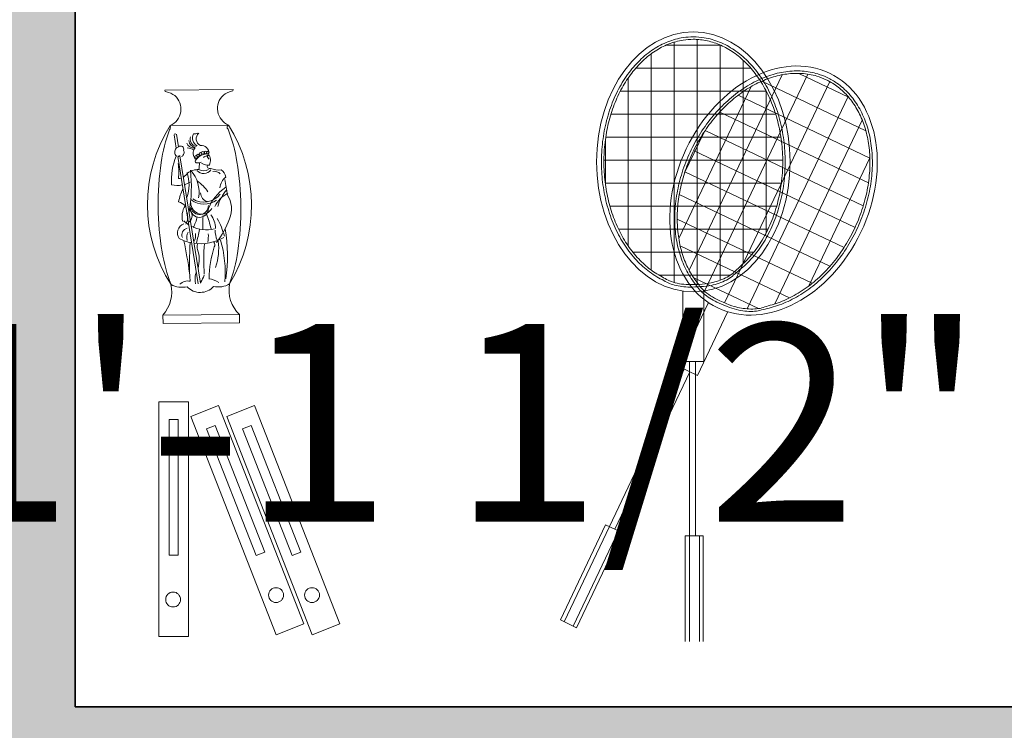
# Model space of a CAD drawing. Units: inches. Extents: x 638 to 1303, y 1 to 699.
# Tile 14 of 21: x 924 to 964, y 548 to 577. Entities that reach past the tile are written whole.
import ezdxf

# ---------------------------------------------------------------- set-up
doc = ezdxf.new("R2010")
doc.units = ezdxf.units.IN
doc.header["$MEASUREMENT"] = 0
for name, color, linetype, lineweight in [('A-ANNO-DIMS', 2, 'Continuous', 18), ('A-FURN-ACCS', 8, 'Continuous', 13), ('A-WALL', 7, 'Continuous', 35)]:
    doc.layers.add(name, color=color, linetype=linetype, lineweight=lineweight)
doc.layers.add('A-WALL-PATT', color=143, linetype='Continuous', lineweight=13, true_color=0x7aafdf)
doc.styles.get("Standard").update_dxf_attribs({"font": 'arial.ttf'})
doc.dimstyles.get("Standard").update_dxf_attribs({"dimtxt": 8, "dimasz": 0.18, "dimexe": 0.18, "dimexo": 0.0625, "dimgap": 0.09, "dimtad": 0, "dimtih": 1, "dimtoh": 1, "dimdec": 4, "dimzin": 0, "dimdsep": 46, "dimlunit": 3, "dimtxsty": 'Standard', "dimcen": 0.09, "dimadec": 0, "dimazin": 0, "dimtfac": 1, "dimtdec": 4, "dimtofl": 0, "dimtmove": 0, "dimatfit": 3, "dimfxl": 1, "dimtolj": 1, "dimtzin": 0, "dimarcsym": 0})

# ---------------------------------------------------------------- blocks, each defined once
blk = doc.blocks.new('*D68')
at = {"layer": 'A-ANNO-DIMS', "color": 0, "lineweight": -2, "transparency": 16777216}
for p, q in [((908.943, 524.881), (908.943, 560.499)), ((909.123, 560.319), (922.058, 560.319)), ((922.238, 524.881), (922.238, 560.499)), ((922.238, 560.319), (922.418, 560.319))]:
    blk.add_line(p, q, dxfattribs=at)
at = {"layer": 'A-ANNO-DIMS', "color": 0, "transparency": 16777216}
for points in [[(909.123, 560.349), (909.123, 560.289), (908.943, 560.319)], [(922.058, 560.349), (922.058, 560.289), (922.238, 560.319)]]:
    blk.add_solid(points, dxfattribs=at)
at = {"layer": 'Defpoints', "color": 0, "transparency": 16777216}
for p in [(922.238, 560.319), (908.943, 524.819), (922.238, 524.819)]:
    blk.add_point(p, dxfattribs=at)
at = {"layer": 'A-ANNO-DIMS', "color": 0, "transparency": 16777216, "insert": (942.085, 560.319), "char_height": 8, "attachment_point": 5}
blk.add_mtext('\\A1;1\'-1 1/2"', dxfattribs=at)

msp = doc.modelspace()

# ---------------------------------------------------------------- hatches: boundary and pattern name
at = {"layer": 'A-WALL-PATT'}
h = msp.add_hatch(color=256, dxfattribs=at)
h.dxf.hatch_style = 1
h.paths.add_polyline_path([(973.34524, 629.81895), (793.35541, 629.81895), (793.35541, 620.81895), (850.23798, 620.81895), (922.23798, 620.81895), (922.23798, 524.81895), (908.94335, 524.81895), (908.94335, 520.31895), (926.73798, 520.31895), (926.73798, 544.31895), (979.3571, 544.31895), (979.3571, 548.81895), (926.73798, 548.81895), (926.73798, 620.81895), (973.34524, 620.81895)])
h.paths.add_polyline_path([(758.35541, 629.81895), (697.23798, 629.81895), (697.23798, 586.77451), (706.23798, 586.77451), (706.23798, 620.81895), (758.35541, 620.81895)])
h.paths.add_polyline_path([(1075.85281, 629.81895), (1003.34524, 629.81895), (1003.34524, 620.81895), (1046.73798, 620.81895), (1046.73798, 560.81895), (1046.73798, 548.81895), (1026.3571, 548.81895), (1026.3571, 544.31895), (1046.73798, 544.31895), (1046.73798, 486.87457), (1051.23798, 486.87457), (1051.23798, 556.31895), (1162.89753, 556.31895), (1162.89753, 560.81895), (1051.23798, 560.81895), (1051.23798, 620.81895), (1075.85281, 620.81895)])
h.paths.add_polyline_path([(1228.23798, 629.81895), (1105.85281, 629.81895), (1105.85281, 620.81895), (1219.23798, 620.81895), (1219.23798, 560.81895), (1197.89753, 560.81895), (1197.89753, 556.31895), (1219.23798, 556.31895), (1219.23798, 498.80084), (1228.23798, 498.80084)])
h.paths.add_polyline_path([(1051.23798, 439.87457), (1046.73798, 439.87457), (1046.73798, 407.81895), (1219.23798, 407.81895), (1219.23798, 381.66175), (1228.23798, 381.66175), (1228.23798, 451.80084), (1219.23798, 451.80084), (1219.23798, 412.31895), (1051.23798, 412.31895)])
h.paths.add_polyline_path([(1228.23798, 346.66175), (1219.23798, 346.66175), (1219.23798, 335.81895), (1046.73798, 335.81895), (1046.73798, 273.56895), (1051.23798, 273.56895), (1051.23798, 331.31895), (1219.23798, 331.31895), (1219.23798, 308.99654), (1228.23798, 308.99654)])
h.paths.add_polyline_path([(1228.23798, 261.99654), (1219.23798, 261.99654), (1219.23798, 211.31895), (1051.23798, 211.31895), (1051.23798, 226.56895), (1046.73798, 226.56895), (1046.73798, 211.31895), (983.84714, 211.31895), (983.84714, 206.81895), (1219.23798, 206.81895), (1219.23798, 166.83987), (1228.23798, 166.83987)])
h.paths.add_polyline_path([(1228.23798, 119.83987), (1219.23798, 119.83987), (1219.23798, 50.81895), (1197.89277, 50.81895), (1197.89277, 41.81895), (1228.23798, 41.81895)])
h.paths.add_polyline_path([(1162.89277, 50.81895), (1069.02949, 50.81895), (1069.02949, 41.81895), (1162.89277, 41.81895)])
h.paths.add_polyline_path([(1010.02949, 50.81895), (941.89631, 50.81895), (917.77455, 50.81895), (917.77455, 41.81895), (941.89631, 41.81895), (1010.02949, 41.81895)])
h.paths.add_polyline_path([(882.77455, 50.81895), (854.73798, 50.81895), (854.73798, 145.50379), (850.23798, 145.50379), (850.23798, 50.81895), (793.49755, 50.81895), (793.49755, 41.81895), (882.77455, 41.81895)])
h.paths.add_polyline_path([(746.49755, 50.81895), (706.23798, 50.81895), (706.23798, 96.57416), (697.23798, 96.57416), (697.23798, 41.81895), (746.49755, 41.81895)])
h.paths.add_polyline_path([(706.23798, 206.81895), (714.01165, 206.81895), (714.01165, 211.31895), (706.23798, 211.31895), (706.23798, 251.21966), (697.23798, 251.21966), (697.23798, 143.57416), (706.23798, 143.57416)])
h.paths.add_polyline_path([(923.84714, 211.31895), (854.73798, 211.31895), (854.73798, 397.8313), (850.23798, 397.8313), (850.23798, 388.31895), (747.9539, 388.31895), (747.9539, 383.81895), (850.23798, 383.81895), (850.23798, 311.81895), (706.23798, 311.81895), (706.23798, 342.78787), (697.23798, 342.78787), (697.23798, 281.21966), (706.23798, 281.21966), (706.23798, 307.31895), (850.23798, 307.31895), (850.23798, 211.31895), (749.01165, 211.31895), (749.01165, 206.81895), (850.23798, 206.81895), (850.23798, 192.50379), (854.73798, 192.50379), (854.73798, 206.81895), (923.84714, 206.81895)])
h.paths.add_polyline_path([(706.23798, 434.70471), (697.23798, 434.70471), (697.23798, 372.78787), (706.23798, 372.78787), (706.23798, 383.81895), (712.9539, 383.81895), (712.9539, 388.31895), (706.23798, 388.31895)])
h.paths.add_polyline_path([(706.23798, 520.31895), (850.23798, 520.31895), (850.23798, 444.8313), (854.73798, 444.8313), (854.73798, 520.31895), (861.94335, 520.31895), (861.94335, 524.81895), (706.23798, 524.81895), (706.23798, 551.77451), (697.23798, 551.77451), (697.23798, 481.70471), (706.23798, 481.70471)])

# ---------------------------------------------------------------- linework, layer by layer
at = {"layer": 'A-FURN-ACCS'}
for p, q in [((951.92482, 565.92116), (951.92482, 575.84384)), ((952.88104, 575.60577), (950.65092, 575.60577)), ((950.9947, 566.0011), (950.9947, 575.73391)), ((952.85493, 566.09836), (952.85493, 575.61728)), ((950.06458, 566.50307), (950.06458, 575.26317)), ((953.78505, 566.76477), (953.78505, 575.00102)), ((954.09923, 574.67566), (949.43274, 574.67566)), ((949.13447, 567.4772), (949.13447, 574.28904)), ((951.5981, 566.50206), (955.36223, 574.41221)), ((952.22228, 565.64913), (956.40438, 574.43761)), ((958.05264, 573.51137), (956.03889, 574.46963)), ((930.36629, 573.79273, 3.93985), (933.1319, 573.82098, 3.93985)), ((951.1768, 567.78134), (954.10378, 573.93226)), ((953.0278, 565.17728), (957.29149, 574.13722)), ((958.75298, 572.14805), (954.53924, 574.1532)), ((954.7224, 573.74554), (948.80958, 573.74554)), ((958.91602, 571.04041), (953.57688, 573.58109)), ((953.94381, 564.93762), (958.03401, 573.53297)), ((954.71517, 568.00675), (954.71517, 573.75949)), ((955.10079, 572.81542), (948.4312, 572.81542)), ((958.85803, 570.03795), (952.83555, 572.90381)), ((955.07004, 565.13971), (958.60908, 572.57684)), ((932.94155, 572.37729, 3.93985), (930.58608, 572.35324, 3.93985)), ((930.73828, 572.00632, 3.93985), (930.81707, 572.02686, 3.93985)), ((930.73848, 571.98658, 3.93985), (930.82557, 571.44523, 3.93985)), ((930.83702, 572.00733, 3.93985), (930.92035, 571.48941, 3.93985)), ((948.20435, 569.98468), (948.20435, 571.78156)), ((955.31279, 571.88531), (948.21919, 571.88531)), ((951.41437, 570.44519), (952.18647, 572.06773)), ((958.6498, 569.10698), (952.24445, 572.15503)), ((930.94371, 571.51169, 3.93985), (930.91472, 571.52437, 3.93985)), ((930.88613, 571.1049, 3.93985), (931.71527, 565.95114, 3.93985)), ((930.97802, 571.13095, 3.93985), (931.80716, 565.9772, 3.93985)), ((958.31746, 568.23507), (951.77746, 571.3472)), ((956.44358, 565.86153), (958.91548, 571.05612)), ((955.38734, 570.95519), (948.14463, 570.95519)), ((957.86867, 567.41857), (951.42692, 570.48395)), ((955.33294, 570.02507), (948.19903, 570.02507)), ((957.29791, 566.66012), (951.19835, 569.56266)), ((955.14346, 569.09496), (948.38851, 569.09496)), ((956.58277, 565.97037), (951.11417, 568.57266)), ((954.79409, 568.16484), (948.73789, 568.16484)), ((955.66331, 565.37785), (951.2343, 567.48544)), ((954.21843, 567.23473), (949.31353, 567.23473)), ((953.27128, 566.30461), (950.36758, 566.30461)), ((954.40839, 564.94496), (951.78642, 566.19265)), ((951.33596, 565.63601), (951.33596, 562.79817)), ((952.19601, 565.63601), (952.19601, 562.79817)), ((952.37355, 565.17282), (951.15416, 562.61032)), ((930.28799, 564.68019, 3.93985), (933.39058, 564.71188, 3.93985)), ((930.28799, 564.68019, 3.93985), (930.29148, 564.33761, 3.93985)), ((933.39058, 564.71188, 3.93985), (933.39408, 564.3693, 3.93985)), ((953.15016, 564.80327), (951.93076, 562.24076)), ((930.29148, 564.33761, 3.93985), (933.39408, 564.3693, 3.93985)), ((951.15416, 562.61032), (951.93076, 562.24076)), ((951.33596, 562.79817), (952.19601, 562.79817)), ((951.60659, 562.79817), (951.60659, 555.74243)), ((951.85462, 562.79817), (951.85462, 555.74243)), ((951.39853, 562.49403), (948.36675, 556.12287)), ((951.6225, 562.38745), (948.59071, 556.01629)), ((930.11865, 551.67657), (930.11865, 561.1656)), ((930.11865, 561.1656), (931.32767, 561.1656)), ((931.32767, 561.1656), (931.32767, 551.67657)), ((931.41319, 560.57978), (932.53902, 561.02049)), ((932.53902, 561.02049), (935.99798, 552.18435)), ((932.87056, 560.57978), (933.99639, 561.02049)), ((933.99639, 561.02049), (937.45534, 552.18435)), ((930.91023, 560.46272), (930.53474, 560.46272)), ((930.53474, 560.46272), (930.53474, 554.96154)), ((930.91023, 554.96154), (930.91023, 560.46272)), ((934.87215, 551.74364), (931.41319, 560.57978)), ((932.40652, 560.21381), (932.05687, 560.07693)), ((934.41182, 555.09114), (932.40652, 560.21381)), ((936.32951, 551.74364), (932.87056, 560.57978)), ((933.86389, 560.21381), (933.51424, 560.07693)), ((935.86919, 555.09114), (933.86389, 560.21381)), ((932.05687, 560.07693), (934.06217, 554.95426)), ((933.51424, 560.07693), (935.51953, 554.95426)), ((946.38188, 552.34124), (948.21563, 556.19478)), ((948.36675, 556.12287), (946.533, 552.26932)), ((948.74148, 555.94455), (946.90773, 552.09101)), ((948.87502, 555.881), (947.04127, 552.02746)), ((948.21563, 556.19478), (948.87502, 555.881)), ((951.43923, 555.74243), (952.16948, 555.74243)), ((951.43923, 551.47483), (951.43923, 555.74243)), ((951.60659, 555.74243), (951.60659, 551.47483)), ((952.02159, 555.74243), (952.02159, 551.47483)), ((952.16948, 555.74243), (952.16948, 551.47483)), ((934.06217, 554.95426), (934.41182, 555.09114)), ((935.51953, 554.95426), (935.86919, 555.09114)), ((930.53474, 554.96154), (930.91023, 554.96154)), ((947.04127, 552.02746), (946.38188, 552.34124)), ((935.99798, 552.18435), (934.87215, 551.74364)), ((937.45534, 552.18435), (936.32951, 551.74364)), ((931.32767, 551.67657), (930.11865, 551.67657))]:
    msp.add_line(p, q, dxfattribs=at)
for centre, radius in [((931.63494, 571.08741, 3.93985), 0.05363), ((931.70144, 571.13832, 3.93985), 0.05363), ((931.80966, 571.20641, 3.93985), 0.05363), ((931.90138, 571.24921, 3.93985), 0.05363), ((932.01849, 571.26715, 3.93985), 0.05363), ((932.10234, 571.25963, 3.93985), 0.05363), ((930.70162, 553.16949), 0.30075), ((934.87081, 553.34635), 0.30075), ((936.32817, 553.34635), 0.30075)]:
    msp.add_circle(centre, radius, dxfattribs=at)
for centre, radius, start, end in [((930.4364, 573.78534, 3.93985), 0.0705, 173.978672, 263.589878), ((933.06195, 573.81215, 3.93985), 0.0705, 277.580483, 7.191689), ((930.28491, 572.92087, 3.93985), 0.80729, 53.36252, 79.752247), ((930.28893, 573.01851, 3.93985), 0.72862, 294.068985, 49.030396), ((933.22506, 573.0485, 3.93985), 0.72862, 132.139965, 247.101376), ((933.23107, 572.95097, 3.93985), 0.80729, 101.418114, 127.807841), ((935.62317, 569.16134, 3.93985), 5.96326, 147.63841, 212.934069), ((936.80547, 569.89792, 3.93985), 6.65759, 159.879075, 171.686697), ((930.38882, 572.30571, 3.93985), 0.20291, 324.592438, 13.5447), ((932.97842, 572.28989, 3.93985), 0.09486, 112.872738, 234.825052), ((926.72059, 569.79492, 3.93985), 6.65759, 9.483664, 21.291286), ((927.75237, 569.1267, 3.93985), 6.12323, 328.676594, 32.063754), ((931.69522, 571.8088, 3.93985), 0.30225, 161.219878, 257.602502), ((931.87895, 571.86156, 3.93985), 0.38896, 155.032994, 237.440628), ((931.5612, 572.48064, 3.93985), 0.45624, 265.618389, 288.22447), ((931.92349, 571.82059, 3.93985), 0.28985, 128.416535, 246.44791), ((930.98098, 571.28762, 3.93985), 0.21579, 135.652185, 231.313321), ((930.95315, 571.29534, 3.93985), 0.19683, 97.608952, 133.084254), ((930.98098, 571.28762, 3.93985), 0.21579, 106.065257, 106.543427), ((931.00569, 571.40497, 3.93985), 0.12341, 338.05295, 133.167285), ((931.53171, 571.7458, 3.93985), 0.29475, 199.396632, 277.795371), ((931.12423, 570.46778, 3.93985), 0.99454, 65.731284, 81.253778), ((931.64392, 571.7836, 3.93985), 0.31433, 186.612201, 260.351866), ((931.82188, 571.23685, 3.93985), 0.31662, 136.70467, 233.998908), ((931.8405, 571.24917, 3.93985), 0.30747, 355.07693, 96.129443), ((933.14517, 570.15203, 3.93985), 2.51236, 157.363881, 184.555163), ((930.97993, 571.0325, 3.93985), 0.09847, 89.36162, 156.718708), ((930.95336, 571.26832, 3.93985), 0.18978, 298.454265, 28.490298), ((932.07819, 570.66237, 3.93985), 0.54504, 82.744379, 144.264353), ((932.06575, 570.9381, 3.93985), 0.1872, 91.201601, 137.200919), ((932.11675, 571.07969, 3.93985), 0.07704, 68.214429, 135.562268), ((934.51128, 572.6537, 3.93985), 2.88286, 211.821697, 215.192011), ((932.05964, 571.22938, 3.93985), 0.10415, 271.201601, 317.867143), ((931.73216, 570.94371, 3.93985), 0.47858, 337.12838, 33.987651), ((941.79914, 569.16824, 3.93985), 11.70429, 171.686697, 180.58518), ((928.6136, 570.49435, 3.93985), 2.31828, 353.001994, 8.168367), ((931.72075, 569.84872, 3.93985), 0.72718, 88.448153, 126.557118), ((931.6521, 570.90935, 3.93985), 0.06058, 93.166791, 258.408226), ((931.70503, 571.17964, 3.93985), 0.33601, 258.827884, 292.582513), ((929.04284, 571.05801, 3.93985), 2.74039, 349.861746, 355.669622), ((931.93491, 570.87411, 3.93985), 0.35624, 236.915164, 304.255197), ((932.09995, 571.15217, 3.93985), 0.4012, 232.608356, 280.506503), ((932.18004, 570.71116, 3.93985), 0.09734, 151.975277, 290.43311), ((932.53204, 571.39072, 3.93985), 0.8338, 247.578924, 278.070792), ((921.74286, 568.96339, 3.93985), 11.70429, 0.58518, 9.483664), ((930.88011, 570.6955, 3.93985), 0.48483, 274.080429, 286.872559), ((930.88011, 570.6955, 3.93985), 0.48483, 299.139964, 327.195908), ((929.80227, 569.96272, 3.93985), 1.54504, 340.445867, 18.476457), ((925.46117, 569.90469, 3.93985), 5.97893, 349.800704, 6.219849), ((930.4197, 569.65847, 3.93985), 1.3323, 350.156464, 41.022084), ((931.93771, 570.78096, 3.93985), 0.36935, 221.679853, 323.437905), ((932.36689, 570.15732, 3.93985), 0.34925, 45.606962, 98.715113), ((933.20294, 569.79199, 3.93985), 0.60711, 127.916667, 176.002542), ((932.3963, 570.20722, 3.93985), 0.43822, 8.360591, 54.769096), ((930.85946, 571.10517, 3.93985), 1.17323, 259.256302, 280.143751), ((932.96614, 568.90138, 3.93985), 2.07389, 154.648215, 169.915004), ((930.85946, 571.10517, 3.93985), 1.17323, 285.066545, 296.896447), ((932.96614, 568.90138, 3.93985), 2.07389, 148.73, 150.009002), ((930.9778, 568.99161, 3.93985), 1.31647, 31.087903, 57.454033), ((933.82022, 568.33727, 3.93985), 1.81119, 122.987839, 160.524595), ((925.12396, 568.56865, 3.93985), 7.83324, 7.132694, 11.809959), ((931.94586, 570.07943, 3.93985), 0.82432, 236.908555, 322.51085), ((932.19048, 569.64425, 3.93985), 0.38143, 182.310148, 254.645077), ((933.51177, 568.50799, 3.93985), 1.26216, 118.1905, 152.943875), ((934.24623, 568.57152, 3.93985), 1.81371, 139.135045, 163.609661), ((932.00236, 568.98323, 3.93985), 1.06448, 337.449397, 32.874556), ((941.79914, 569.16824, 3.93985), 11.70429, 180.58518, 189.483664), ((930.68518, 568.5214, 3.93985), 0.78066, 48.563779, 72.163918), ((931.89881, 568.68176, 3.93985), 0.83406, 149.165045, 194.233015), ((931.76637, 569.00441, 3.93985), 0.36546, 181.777586, 359.392726), ((931.87408, 569.22743, 3.93985), 0.45567, 179.662937, 330.34047), ((931.77093, 569.11359, 3.93985), 0.3597, 192.9887, 0.854117), ((931.95684, 570.04499, 3.93985), 0.86894, 233.251607, 305.716721), ((921.74286, 568.96339, 3.93985), 11.70429, 351.686697, 0.58518), ((930.71438, 568.65661, 3.93985), 0.5779, 329.05964, 17.851904), ((931.1593, 568.70439, 3.93985), 0.31379, 302.464066, 58.706295), ((929.79658, 569.15693, 3.93985), 1.94875, 331.409171, 345.237839), ((937.06034, 568.31067, 3.93985), 5.15937, 175.427248, 181.790816), ((927.14768, 566.96975, 3.93985), 5.2315, 13.292723, 20.275302), ((931.38178, 568.15557, 3.93985), 1.0355, 2.135398, 34.693756), ((929.56809, 567.00685, 3.93985), 3.32443, 15.262978, 28.432739), ((931.27385, 568.00443, 3.93985), 0.40039, 110.925785, 213.353073), ((931.33295, 567.93208, 3.93985), 0.27715, 102.936106, 202.6875), ((932.05356, 569.49529, 3.93985), 1.36035, 227.22056, 237.889319), ((932.05356, 569.49529, 3.93985), 1.36035, 243.009854, 283.765708), ((929.0917, 570.0943, 3.93985), 4.17966, 323.739259, 338.684771), ((931.81216, 569.49248, 3.93985), 1.91823, 242.936433, 259.073084), ((931.59793, 567.8441, 3.93985), 0.34926, 144.945369, 202.796846), ((931.14157, 567.91686, 3.93985), 0.47275, 325.954787, 8.718551), ((931.81216, 569.49248, 3.93985), 1.91823, 262.062534, 299.478659), ((-1212959.28846, 247911.29423, 3.93985), 1238834.17867, 348.48301372545, 348.48303986891), ((930.94009, 567.86326, 3.93985), 1.18763, 349.081374, 5.351792), ((933.76784, 568.1981, 3.93985), 1.37275, 183.470149, 200.333874), ((926.50054, 567.09745, 3.93985), 6.40311, 351.45087, 9.71949), ((909.96653, 563.26358, 3.93985), 21.62867, 8.303796, 11.802898), ((941.70043, 566.81783, 3.93985), 10.33722, 175.488003, 184.249156), ((931.97939, 567.44949, 3.93985), 0.30591, 159.799983, 201.370377), ((940.3671, 566.90825, 3.93985), 8.42516, 175.44269, 183.907751), ((936.68024, 566.09932, 3.93985), 4.51979, 162.697804, 179.250289), ((932.23917, 567.52946, 3.93985), 0.15233, 325.674824, 46.923716), ((930.45468, 567.35144, 3.93985), 2.09214, 339.390871, 9.091232), ((928.17324, 566.40591, 3.93985), 4.6365, 355.309359, 16.496738), ((936.82141, 568.33671, 3.93985), 6.65759, 189.483664, 201.291286), ((930.47506, 566.93868, 3.93985), 1.28317, 344.089179, 18.132248), ((926.73654, 568.2337, 3.93985), 6.65759, 339.879075, 351.686697), ((932.34974, 566.13539, 3.93985), 0.76143, 162.04486, 193.669528), ((930.47506, 566.93868, 3.93985), 1.28317, 333.698527, 335.445092), ((83932.43772, -39905.60547, 3.93985), 92342.04718, 154.0056530881, 154.0058448081), ((929.20436, 565.6302, 3.93985), 1.4411, 318.759111, 12.038114), ((931.06593, 566.75648, 3.93985), 0.9494, 241.863974, 282.544569), ((931.28714, 565.64577, 3.93985), 0.41937, 75.573225, 137.468871), ((931.79904, 566.32053, 3.93985), 0.72006, 222.967172, 270.58518), ((931.79904, 566.32053, 3.93985), 0.72006, 270.58518, 318.203188), ((931.96493, 565.04008, 3.93985), 1.13197, 58.43802, 81.047436), ((932.52309, 566.77137, 3.93985), 0.9494, 258.625792, 299.306386), ((934.28094, 565.68472, 3.93985), 1.31878, 168.684615, 227.534507)]:
    msp.add_arc(centre, radius, start, end, dxfattribs=at)
for centre, major_axis in [((951.76598, 570.88312), (0, 5.26318)), ((955.01649, 569.72606), (2.26154, 4.75252))]:
    msp.add_ellipse(centre, major_axis=major_axis, ratio=0.74468092, dxfattribs=at)
for points, knots in [([(951.76598, 575.94787), (951.62974, 575.94787), (951.49349, 575.93763), (951.1486, 575.88559), (950.94092, 575.82962), (950.53439, 575.66984), (950.33554, 575.56603), (949.95255, 575.31279), (949.76842, 575.16336), (949.42077, 574.82271), (949.25727, 574.6315), (948.95634, 574.21275), (948.81892, 573.98521), (948.57479, 573.50061), (948.46809, 573.24356), (948.28899, 572.70779), (948.21659, 572.42908), (948.10851, 571.85858), (948.07283, 571.5668), (948.03938, 570.9792), (948.04161, 570.68338), (948.0839, 570.09684), (948.12397, 569.80614), (948.2406, 569.23881), (948.31717, 568.96221), (948.50424, 568.4316), (948.61475, 568.17762), (948.86599, 567.70001), (949.00672, 567.4764), (949.31367, 567.06622), (949.47989, 566.87965), (949.83228, 566.54882), (950.01844, 566.40456), (950.4048, 566.16201), (950.60498, 566.06372), (950.8895, 565.91514), (951.09784, 565.86485), (951.51726, 565.81308), (951.72835, 565.8116), (952.39612, 565.85745), (952.60478, 565.9048), (953.01428, 566.04756), (953.21512, 566.14299), (953.47914, 566.37997), (953.66633, 566.52152), (954.02111, 566.84722), (954.1887, 567.03136), (954.49872, 567.43705), (954.64114, 567.65859), (954.89602, 568.13249), (955.00848, 568.38484), (955.19965, 568.91268), (955.27835, 569.18815), (955.39939, 569.75374), (955.44172, 570.04384), (955.48859, 570.62973), (955.49313, 570.9255), (955.46427, 571.51356), (955.43087, 571.80584), (955.32724, 572.37788), (955.25701, 572.65764), (955.08206, 573.196), (954.97735, 573.4546), (954.73695, 573.94274), (954.60127, 574.17227), (954.30352, 574.59539), (954.14145, 574.78897), (953.79632, 575.13466), (953.61327, 575.28675), (953.23209, 575.5455), (953.03396, 575.65216), (952.62853, 575.81771), (952.42122, 575.87662), (952.064, 575.93562), (951.91499, 575.94787), (951.76598, 575.94787)], [0, 0, 0, 0, 0.11189338, 0.11189338, 0.2847196, 0.2847196, 0.45754582, 0.45754582, 0.63037204, 0.63037204, 0.80319826, 0.80319826, 0.97602448, 0.97602448, 1.1488507, 1.1488507, 1.32167692, 1.32167692, 1.49450315, 1.49450315, 1.66732937, 1.66732937, 1.84015559, 1.84015559, 2.01298181, 2.01298181, 2.18580803, 2.18580803, 2.35863425, 2.35863425, 2.53146047, 2.53146047, 2.70428669, 2.70428669, 2.87711291, 2.87711291, 3.04993914, 3.04993914, 3.22276536, 3.22276536, 3.39559158, 3.39559158, 3.5684178, 3.5684178, 3.74124402, 3.74124402, 3.91407024, 3.91407024, 4.08689646, 4.08689646, 4.25972268, 4.25972268, 4.4325489, 4.4325489, 4.60537513, 4.60537513, 4.77820135, 4.77820135, 4.95102757, 4.95102757, 5.12385379, 5.12385379, 5.29668001, 5.29668001, 5.46950623, 5.46950623, 5.64233245, 5.64233245, 5.81515867, 5.81515867, 5.98798489, 5.98798489, 6.16081112, 6.16081112, 6.28318531, 6.28318531, 6.28318531, 6.28318531]), ([(951.76598, 575.84866), (951.63014, 575.84866), (951.49428, 575.8381), (951.15487, 575.78508), (950.95211, 575.72907), (950.57178, 575.57625), (950.39349, 575.48331), (950.04801, 575.25882), (949.88081, 575.12714), (949.56253, 574.82786), (949.41145, 574.66018), (949.12993, 574.29282), (948.99952, 574.09308), (948.76333, 573.66667), (948.6576, 573.43996), (948.47399, 572.96557), (948.39616, 572.71789), (948.27076, 572.20818), (948.22321, 571.94619), (948.15981, 571.41491), (948.14398, 571.14568), (948.14452, 570.60723), (948.16087, 570.33805), (948.22532, 569.80702), (948.27337, 569.5452), (948.39978, 569.03597), (948.47808, 568.78858), (948.66261, 568.31489), (948.76878, 568.08857), (949.00578, 567.66306), (949.13658, 567.4638), (949.41877, 567.0975), (949.57017, 566.93039), (949.88724, 566.6339), (950.05278, 566.50408), (950.40991, 566.27253), (950.60254, 566.17427), (950.9059, 566.01083), (951.1421, 565.95457), (951.617, 565.90691), (952.1038, 565.91547), (952.53766, 565.99058), (952.73343, 566.04727), (953.11719, 566.20525), (953.30515, 566.30649), (953.54391, 566.55192), (953.7187, 566.69604), (954.04949, 567.02396), (954.20549, 567.20769), (954.49341, 567.60989), (954.62534, 567.82831), (954.86058, 568.2936), (954.96392, 568.54043), (955.13843, 569.05519), (955.20965, 569.3231), (955.3175, 569.87195), (955.35418, 570.15289), (955.39171, 570.71927), (955.39261, 571.00475), (955.35858, 571.57156), (955.32368, 571.85293), (955.2208, 572.3947), (955.15388, 572.65552), (954.98989, 573.15701), (954.89291, 573.39781), (954.67348, 573.85024), (954.55138, 574.06228), (954.28751, 574.45158), (954.14618, 574.62945), (953.84613, 574.95173), (953.6874, 575.09607), (953.35702, 575.34827), (953.1854, 575.45606), (952.83368, 575.63339), (952.65363, 575.70288), (952.28907, 575.80283), (952.1046, 575.8333), (951.86846, 575.84716), (951.81722, 575.84866), (951.76598, 575.84866)], [0, 0, 0, 0, 0.11579064, 0.11579064, 0.29073032, 0.29073032, 0.4507067, 0.4507067, 0.61090847, 0.61090847, 0.77111024, 0.77111024, 0.93131201, 0.93131201, 1.09151378, 1.09151378, 1.25171555, 1.25171555, 1.41191732, 1.41191732, 1.57211909, 1.57211909, 1.73232086, 1.73232086, 1.89252263, 1.89252263, 2.0527244, 2.0527244, 2.21292617, 2.21292617, 2.37312794, 2.37312794, 2.53332971, 2.53332971, 2.69180105, 2.69180105, 2.86418207, 2.86418207, 3.06698542, 3.06698542, 3.26978878, 3.26978878, 3.43901445, 3.43901445, 3.60824012, 3.60824012, 3.77746579, 3.77746579, 3.94669146, 3.94669146, 4.11591713, 4.11591713, 4.2851428, 4.2851428, 4.45436847, 4.45436847, 4.62359414, 4.62359414, 4.79281981, 4.79281981, 4.96204548, 4.96204548, 5.12614683, 5.12614683, 5.28969056, 5.28969056, 5.45084761, 5.45084761, 5.60858038, 5.60858038, 5.76631316, 5.76631316, 5.92404593, 5.92404593, 6.08177871, 6.08177871, 6.23951149, 6.23951149, 6.28318531, 6.28318531, 6.28318531, 6.28318531]), ([(957.19277, 574.29941), (957.06974, 574.35795), (956.94231, 574.40725), (956.60852, 574.50845), (956.39694, 574.54715), (955.9612, 574.57756), (955.73704, 574.56926), (955.28239, 574.50516), (955.05191, 574.44934), (954.59162, 574.29113), (954.36182, 574.18873), (953.91016, 573.93991), (953.6883, 573.7935), (953.25963, 573.46081), (953.05283, 573.27455), (952.66089, 572.86772), (952.47575, 572.64716), (952.13302, 572.17846), (951.97543, 571.93032), (951.69274, 571.4141), (951.56764, 571.14603), (951.3538, 570.59823), (951.26507, 570.31851), (951.12661, 569.75611), (951.07689, 569.47344), (951.01782, 568.91394), (951.00847, 568.63711), (951.03011, 568.09789), (951.06111, 567.8355), (951.16202, 567.33322), (951.23194, 567.09333), (951.40799, 566.64318), (951.5141, 566.43293), (951.75876, 566.0479), (951.89728, 565.87312), (952.09035, 565.61671), (952.25687, 565.48177), (952.61335, 565.25481), (952.80332, 565.16277), (953.426, 564.91724), (953.63476, 564.87033), (954.06588, 564.82328), (954.28823, 564.82315), (954.62847, 564.92369), (954.85832, 564.97108), (955.31863, 565.11273), (955.54908, 565.20699), (956.00334, 565.4401), (956.22713, 565.57895), (956.66092, 565.89736), (956.8709, 566.0769), (957.27032, 566.47138), (957.45976, 566.68631), (957.81209, 567.14501), (957.97496, 567.38878), (958.26903, 567.89768), (958.40022, 568.1628), (958.62684, 568.70621), (958.72227, 568.98448), (958.8745, 569.54555), (958.93129, 569.82834), (959.00465, 570.38964), (959.02121, 570.66815), (959.01389, 571.21222), (958.99001, 571.47778), (958.90295, 571.98779), (958.83979, 572.23223), (958.67668, 572.69267), (958.57675, 572.90866), (958.34373, 573.3061), (958.21065, 573.48754), (957.91569, 573.81125), (957.75382, 573.95352), (957.45661, 574.16029), (957.32732, 574.23538), (957.19277, 574.29941)], [0, 0, 0, 0, 0.11189338, 0.11189338, 0.2847196, 0.2847196, 0.45754582, 0.45754582, 0.63037204, 0.63037204, 0.80319826, 0.80319826, 0.97602448, 0.97602448, 1.1488507, 1.1488507, 1.32167692, 1.32167692, 1.49450315, 1.49450315, 1.66732937, 1.66732937, 1.84015559, 1.84015559, 2.01298181, 2.01298181, 2.18580803, 2.18580803, 2.35863425, 2.35863425, 2.53146047, 2.53146047, 2.70428669, 2.70428669, 2.87711291, 2.87711291, 3.04993914, 3.04993914, 3.22276536, 3.22276536, 3.39559158, 3.39559158, 3.5684178, 3.5684178, 3.74124402, 3.74124402, 3.91407024, 3.91407024, 4.08689646, 4.08689646, 4.25972268, 4.25972268, 4.4325489, 4.4325489, 4.60537513, 4.60537513, 4.77820135, 4.77820135, 4.95102757, 4.95102757, 5.12385379, 5.12385379, 5.29668001, 5.29668001, 5.46950623, 5.46950623, 5.64233245, 5.64233245, 5.81515867, 5.81515867, 5.98798489, 5.98798489, 6.16081112, 6.16081112, 6.28318531, 6.28318531, 6.28318531, 6.28318531]), ([(957.15014, 574.20982), (957.02747, 574.26819), (956.90025, 574.31703), (956.571, 574.415), (956.36385, 574.45155), (955.95475, 574.47698), (955.75382, 574.46967), (955.3454, 574.4154), (955.13784, 574.36835), (954.72184, 574.23487), (954.51337, 574.14837), (954.10131, 573.93763), (953.89773, 573.8133), (953.50123, 573.52975), (953.30834, 573.37047), (952.9387, 573.021), (952.76201, 572.83079), (952.42975, 572.42443), (952.27424, 572.20828), (951.98871, 571.75579), (951.85873, 571.51948), (951.62784, 571.03305), (951.52695, 570.78296), (951.35696, 570.27576), (951.28785, 570.01869), (951.18319, 569.50456), (951.14759, 569.24752), (951.11068, 568.7405), (951.1093, 568.49052), (951.14046, 568.00445), (951.17295, 567.76833), (951.27036, 567.31631), (951.33527, 567.10036), (951.49418, 566.69639), (951.58788, 566.50804), (951.81086, 566.1455), (951.94258, 565.97399), (952.14628, 565.69607), (952.33538, 565.54377), (952.74372, 565.29668), (953.18697, 565.09523), (953.61101, 564.97663), (953.81215, 564.9437), (954.22656, 564.92145), (954.43978, 564.93211), (954.76084, 565.05113), (954.98059, 565.10616), (955.42019, 565.26013), (955.64001, 565.35899), (956.07281, 565.59846), (956.2858, 565.73899), (956.69814, 566.05806), (956.89752, 566.23653), (957.27628, 566.62637), (957.45571, 566.83768), (957.78893, 567.28694), (957.94276, 567.52486), (958.22003, 568.02017), (958.34351, 568.27755), (958.55633, 568.80399), (958.64572, 569.07306), (958.78561, 569.60647), (958.83726, 569.87074), (958.90467, 570.39405), (958.92057, 570.65315), (958.91683, 571.15598), (958.89769, 571.39991), (958.8267, 571.86481), (958.77551, 572.08616), (958.64306, 572.5061), (958.56174, 572.70463), (958.37179, 573.07433), (958.26314, 573.2454), (958.02174, 573.55665), (957.88902, 573.69677), (957.60278, 573.94368), (957.4493, 574.05045), (957.24203, 574.16443), (957.1964, 574.1878), (957.15014, 574.20982)], [0, 0, 0, 0, 0.11579064, 0.11579064, 0.29073032, 0.29073032, 0.4507067, 0.4507067, 0.61090847, 0.61090847, 0.77111024, 0.77111024, 0.93131201, 0.93131201, 1.09151378, 1.09151378, 1.25171555, 1.25171555, 1.41191732, 1.41191732, 1.57211909, 1.57211909, 1.73232086, 1.73232086, 1.89252263, 1.89252263, 2.0527244, 2.0527244, 2.21292617, 2.21292617, 2.37312794, 2.37312794, 2.53332971, 2.53332971, 2.69180105, 2.69180105, 2.86418207, 2.86418207, 3.06698542, 3.06698542, 3.26978878, 3.26978878, 3.43901445, 3.43901445, 3.60824012, 3.60824012, 3.77746579, 3.77746579, 3.94669146, 3.94669146, 4.11591713, 4.11591713, 4.2851428, 4.2851428, 4.45436847, 4.45436847, 4.62359414, 4.62359414, 4.79281981, 4.79281981, 4.96204548, 4.96204548, 5.12614683, 5.12614683, 5.28969056, 5.28969056, 5.45084761, 5.45084761, 5.60858038, 5.60858038, 5.76631316, 5.76631316, 5.92404593, 5.92404593, 6.08177871, 6.08177871, 6.23951149, 6.23951149, 6.28318531, 6.28318531, 6.28318531, 6.28318531])]:
    msp.add_open_spline(points, degree=3, knots=knots, dxfattribs=at)
at = {"layer": 'A-WALL'}
for p, q in [((926.73798, 548.81895), (926.73798, 620.81895)), ((979.3571, 548.81895), (926.73798, 548.81895))]:
    msp.add_line(p, q, dxfattribs=at)

# ---------------------------------------------------------------- dimensions: what is measured, and where the dimension line sits
at = {"layer": 'A-ANNO-DIMS'}
dim = msp.add_linear_dim(base=(922.23798, 560.31895), p1=(908.94335, 524.81895), p2=(922.23798, 524.81895), angle=0, dimstyle='Standard', override={"dimdec": 1, "dimlfac": 1, "dimrnd": 0, "dimzin": 1, "dimdsep": 46, "dimlunit": 4, "dimfrac": 2}, dxfattribs=at)
dim.commit()
dim.dimension.update_dxf_attribs({"geometry": '*D68', "text_midpoint": (942.08506, 560.31895)})

doc.saveas('drawing.dxf')
